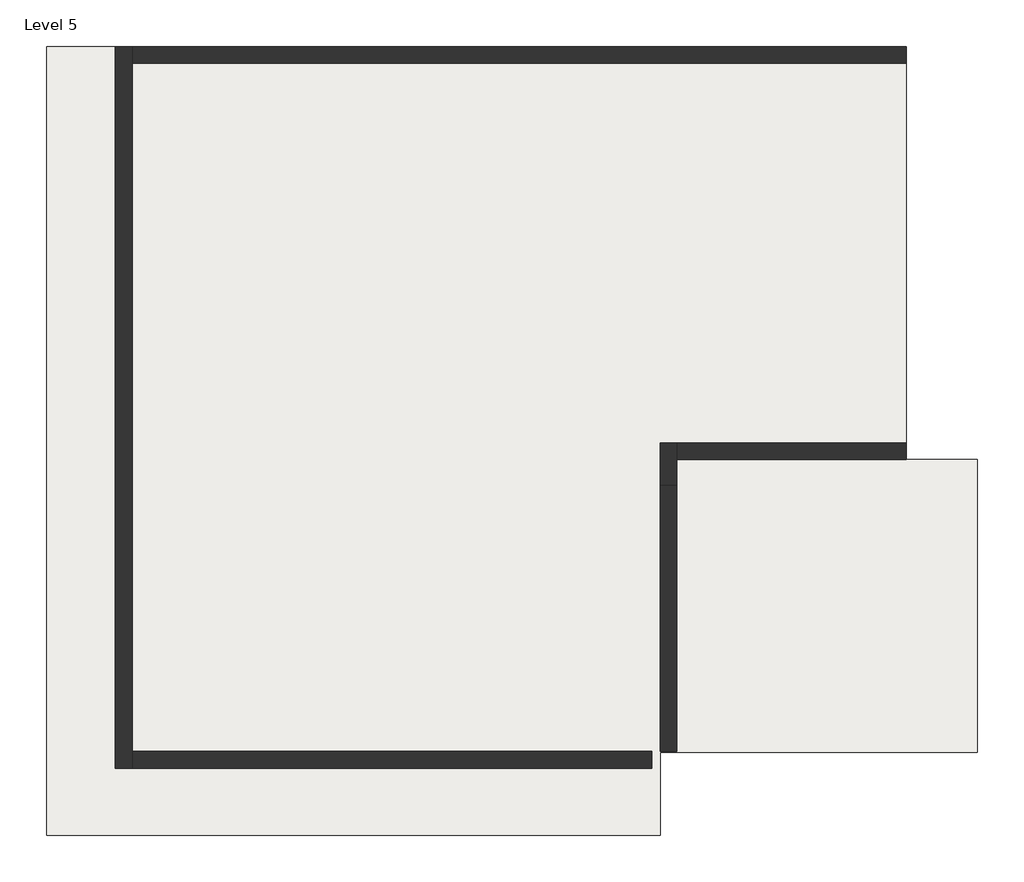
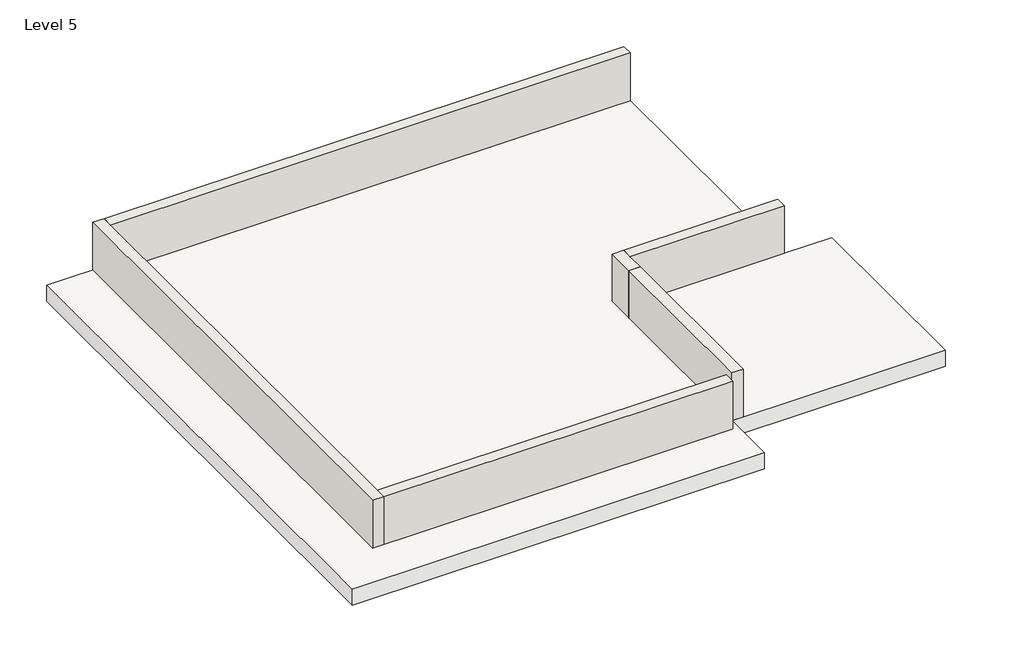
# One storey: 6 walls, 1 roof.
"""IFC4 building model written with IfcOpenShell, lengths in millimetres."""

from ifc_helpers import new_model, si_unit, frame, origin, place, context, project, spatial, polyline, outline, extrude, faceted_brep, element, save

model = new_model("IFC4")

# Units and contexts
model_context = context("Model", 3, world=origin())
ifc_project = project(units=[si_unit("LENGTHUNIT", "METRE", prefix="MILLI")], contexts=[model_context])

# Site, building, storey
site = spatial("IfcSite", under=ifc_project)
building = spatial("IfcBuilding", under=site)
storey = spatial("IfcBuildingStorey", under=building, Name="Level 5", Elevation=14630.4)

# Roof
placement = place(None, origin())
element("IfcRoof", 1, ObjectType="Generic - 12\"", at=placement, inside=storey, context=model_context, shape_type="SweptSolid", body=[
    extrude(outline(polyline([(-4221.3821198, 1549.45098), (-4221.3821198, 539.80098), (-11688.9821198, 539.80098), (-11688.9821198, 10141.00098), (-1224.1821198, 10141.00098), (-1224.1821198, 5111.80098), (-360.5821198, 5111.80098), (-360.5821198, 1549.45098), (-4221.3821198, 1549.45098)])), frame((0.0, 0.0, 14630.4), z_axis=(0.0, 0.0, 1.0), x_axis=(1.0, 0.0, 0.0)), (0.0, 0.0, 1.0), 304.8),
])

# Walls
element("IfcWall", 2, ObjectType="Generic - 8\"", at=placement, inside=storey, context=model_context, shape_type="Brep", body=[
    faceted_brep([(-10647.5821198, 1355.2652184, 14630.4), (-10647.5821198, 1558.4652184, 14630.4), (-10647.5821198, 9937.80098, 14630.4), (-10647.5821198, 10141.00098, 14630.4), (-10647.5821198, 10141.00098, 15849.6), (-10647.5821198, 9937.80098, 15849.6), (-10647.5821198, 1558.4652184, 15849.6), (-10647.5821198, 1355.2652184, 15849.6), (-10850.7821198, 1355.2652184, 14630.4), (-10850.7821198, 1355.2652184, 15849.6), (-10850.7821198, 10141.00098, 15849.6), (-10850.7821198, 10141.00098, 14630.4)], [[[0, 1, 2, 3, 4, 5, 6, 7]], [[8, 9, 10, 11]], [[3, 2, 1, 0, 8, 11]], [[7, 6, 5, 4, 10, 9]], [[0, 7, 9, 8]], [[4, 3, 11, 10]]]),
])
element("IfcWall", 3, ObjectType="Generic - 8\"", at=placement, inside=storey, context=model_context, shape_type="SweptSolid", body=[
    extrude(outline(polyline([(-4221.3821198, 1558.4652184), (-4221.3821198, 4793.9280349), (-4018.1821198, 4793.9280349), (-4018.1821198, 1558.4652184), (-4221.3821198, 1558.4652184)])), frame((0.0, 0.0, 14630.4), z_axis=(0.0, 0.0, 1.0), x_axis=(1.0, 0.0, 0.0)), (0.0, 0.0, 1.0), 1219.2),
])
element("IfcWall", 4, ObjectType="Generic - 8\"", at=placement, inside=storey, context=model_context, shape_type="Brep", body=[
    faceted_brep([(-4322.9821198, 1558.4652184, 14630.4), (-10647.5821198, 1558.4652184, 14630.4), (-10647.5821198, 1558.4652184, 15849.6), (-4322.9821198, 1558.4652184, 15849.6), (-4322.9821198, 1355.2652184, 14630.4), (-4322.9821198, 1355.2652184, 15849.6), (-10647.5821198, 1355.2652184, 15849.6), (-10647.5821198, 1355.2652184, 14630.4), (-4424.5821198, 1355.2652184, 14630.4)], [[[0, 1, 2, 3]], [[4, 5, 6, 7, 8]], [[1, 0, 4, 8, 7]], [[3, 2, 6, 5]], [[0, 3, 5, 4]], [[2, 1, 7, 6]]]),
])
element("IfcWall", 5, ObjectType="Generic - 8\"", at=placement, inside=storey, context=model_context, shape_type="Brep", body=[
    faceted_brep([(-10647.5821198, 9937.80098, 14630.4), (-10114.1821198, 9937.80098, 14630.4), (-1224.1821198, 9937.80098, 14630.4), (-1224.1821198, 9937.80098, 15849.6), (-10647.5821198, 9937.80098, 15849.6), (-10647.5821198, 10141.00098, 14630.4), (-10647.5821198, 10141.00098, 15849.6), (-1224.1821198, 10141.00098, 15849.6), (-1224.1821198, 10141.00098, 14630.4), (-10114.1821198, 10141.00098, 14630.4)], [[[0, 1, 2, 3, 4]], [[5, 6, 7, 8, 9]], [[2, 1, 0, 5, 9, 8]], [[4, 3, 7, 6]], [[0, 4, 6, 5]], [[2, 8, 7, 3]]]),
])
element("IfcWall", 6, ObjectType="Generic - 8\"", at=placement, inside=storey, context=model_context, shape_type="SweptSolid", body=[
    extrude(outline(polyline([(-4018.1821198, 5315.00098), (-1224.1821198, 5315.00098), (-1224.1821198, 5111.80098), (-4018.1821198, 5111.80098), (-4018.1821198, 5315.00098)])), frame((0.0, 0.0, 14630.4), z_axis=(0.0, 0.0, 1.0), x_axis=(1.0, 0.0, 0.0)), (0.0, 0.0, 1.0), 1219.2),
])
element("IfcWall", 7, ObjectType="Generic - 8\"", at=placement, inside=storey, context=model_context, shape_type="Brep", body=[
    faceted_brep([(-4018.1821198, 4793.9280349, 14630.4), (-4018.1821198, 5111.80098, 14630.4), (-4018.1821198, 5315.00098, 14630.4), (-4018.1821198, 5315.00098, 15849.6), (-4018.1821198, 5111.80098, 15849.6), (-4018.1821198, 4793.9280349, 15849.6), (-4221.3821198, 4793.9280349, 14630.4), (-4221.3821198, 4793.9280349, 15849.6), (-4221.3821198, 5315.00098, 15849.6), (-4221.3821198, 5315.00098, 14630.4)], [[[0, 1, 2, 3, 4, 5]], [[6, 7, 8, 9]], [[2, 1, 0, 6, 9]], [[5, 4, 3, 8, 7]], [[0, 5, 7, 6]], [[3, 2, 9, 8]]]),
])

save(model, "model.ifc")

# Revit data of these elements
# Type "Generic - 12\""
#   Assembly Code = "B1020"
#   Layers, outside or top first: 1' - 0" no material (function 1)
# Type "Generic - 8\""
#   Assembly Code = "B2010"
#   Layers, outside or top first: 0' - 8" no material (function 1)
# Element 1 (IfcRoof, "Generic - 12\"")
#   built-in parameter 1001705 = 49 (stored number, unit not read)
#   built-in parameter 1001710 = 33615
#   Phase Created = New Construction
#   Materials on its faces: "Default Roof", "Earth"
# Elements 2, 4 (IfcWall, "Generic - 8\"")
#   Top Offset = 0' - 0"
#   Base Offset = 0' - 0"
#   Unconnected Height = 4' - 0"
#   wall height = 4' - 0"
#   Phase Created = New Construction
#   Base Constraint = Level 5
#   Materials on its faces: "Default Wall", "Tile, Porcelain, 4in"
# Elements 3, 5, 6, 7 (IfcWall, "Generic - 8\"")
#   Top Offset = 0' - 0"
#   Base Offset = 0' - 0"
#   Unconnected Height = 4' - 0"
#   wall height = 4' - 0"
#   Phase Created = New Construction
#   Base Constraint = Level 5
#   Materials on its faces: "Default Wall"
# Materials
#   "Default Roof": colour RGB 88 101 114, transparency 0
#   "Earth": class "Generic", colour RGB 97 75 62, transparency 0, Description = "Soil", Cost = 0
#   "Default Wall": colour RGB 128 128 128, transparency 0
#   "Tile, Porcelain, 4in": class "Generic", colour RGB 89 87 158, transparency 0, Description = "Porcelain tile, 4\", white", Cost = 0
